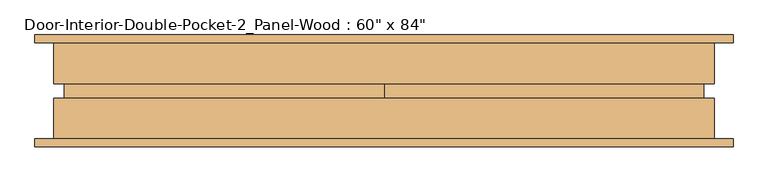
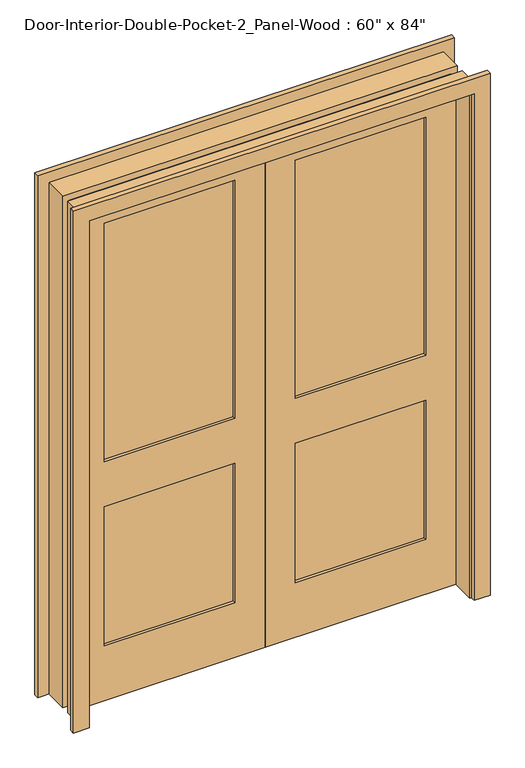
"""IFC4 building model written with IfcOpenShell, lengths in millimetres: door geometry."""

from ifc_helpers import new_model, si_unit, frame, origin, place, context, project, spatial, polyline, outline, extrude, source, transform, mapped, element, save


def door_53d589bd(model_context):
    return source(origin(), model_context, "Body", "SweptSolid", [
        extrude(outline(polyline([(0.0, 768.35), (0.0, 831.85), (2203.45, 831.85), (2203.45, -831.85), (0.0, -831.85), (0.0, -768.35), (2139.95, -768.35), (2139.95, 768.35), (0.0, 768.35)])), frame((0.0, -133.35, 0.0), z_axis=(0.0, 1.0, 0.0), x_axis=(0.0, 0.0, 1.0)), (0.0, 0.0, 1.0), 19.05),
        extrude(outline(polyline([(0.0, 768.35), (0.0, 831.85), (2203.45, 831.85), (2203.45, -831.85), (0.0, -831.85), (0.0, -768.35), (2139.95, -768.35), (2139.95, 768.35), (0.0, 768.35)])), frame((0.0, 114.3, 0.0), z_axis=(0.0, 1.0, 0.0), x_axis=(0.0, 0.0, 1.0)), (0.0, 0.0, 1.0), 19.05),
        extrude(outline(polyline([(-120.65, -5.8208333), (-641.35, -5.8208333), (-641.35, 5.8208333), (-120.65, 5.8208333), (-120.65, -5.8208333)])), frame((0.0, 0.0, 1009.65), z_axis=(0.0, 0.0, 1.0), x_axis=(1.0, 0.0, 0.0)), (0.0, 0.0, 1.0), 1004.8875),
        extrude(outline(polyline([(-120.65, -5.8208333), (-641.35, -5.8208333), (-641.35, 5.8208333), (-120.65, 5.8208333), (-120.65, -5.8208333)])), frame((0.0, 0.0, 231.775), z_axis=(0.0, 0.0, 1.0), x_axis=(1.0, 0.0, 0.0)), (0.0, 0.0, 1.0), 587.375),
        extrude(outline(polyline([(2133.6, -762.0), (0.0, -762.0), (0.0, 0.0), (2133.6, 0.0), (2133.6, -762.0)]), holes=[polyline([(2014.5375, -641.35), (2014.5375, -120.65), (1009.65, -120.65), (1009.65, -641.35), (2014.5375, -641.35)]), polyline([(819.15, -641.35), (819.15, -120.65), (231.775, -120.65), (231.775, -641.35), (819.15, -641.35)])]), frame((0.0, -17.4625, 0.0), z_axis=(0.0, 1.0, 0.0), x_axis=(0.0, 0.0, 1.0)), (0.0, 0.0, 1.0), 34.925),
        extrude(outline(polyline([(0.0, 787.4), (2159.0, 787.4), (2159.0, -787.4), (0.0, -787.4), (0.0, -762.0), (2133.6, -762.0), (2133.6, 762.0), (0.0, 762.0), (0.0, 787.4)])), frame((0.0, 17.4625, 0.0), z_axis=(0.0, 1.0, 0.0), x_axis=(0.0, 0.0, 1.0)), (0.0, 0.0, 1.0), 96.8375),
        extrude(outline(polyline([(0.0, 787.4), (2159.0, 787.4), (2159.0, -787.4), (0.0, -787.4), (0.0, -762.0), (2133.6, -762.0), (2133.6, 762.0), (0.0, 762.0), (0.0, 787.4)])), frame((0.0, -114.3, 0.0), z_axis=(0.0, 1.0, 0.0), x_axis=(0.0, 0.0, 1.0)), (0.0, 0.0, 1.0), 96.8375),
        extrude(outline(polyline([(641.35, -5.8208333), (120.65, -5.8208333), (120.65, 5.8208333), (641.35, 5.8208333), (641.35, -5.8208333)])), frame((0.0, 0.0, 1009.65), z_axis=(0.0, 0.0, 1.0), x_axis=(1.0, 0.0, 0.0)), (0.0, 0.0, 1.0), 1004.8875),
        extrude(outline(polyline([(641.35, -5.8208333), (120.65, -5.8208333), (120.65, 5.8208333), (641.35, 5.8208333), (641.35, -5.8208333)])), frame((0.0, 0.0, 231.775), z_axis=(0.0, 0.0, 1.0), x_axis=(1.0, 0.0, 0.0)), (0.0, 0.0, 1.0), 587.375),
        extrude(outline(polyline([(2133.6, 0.0), (0.0, 0.0), (0.0, 762.0), (2133.6, 762.0), (2133.6, 0.0)]), holes=[polyline([(2014.5375, 120.65), (2014.5375, 641.35), (1009.65, 641.35), (1009.65, 120.65), (2014.5375, 120.65)]), polyline([(819.15, 120.65), (819.15, 641.35), (231.775, 641.35), (231.775, 120.65), (819.15, 120.65)])]), frame((0.0, -17.4625, 0.0), z_axis=(0.0, 1.0, 0.0), x_axis=(0.0, 0.0, 1.0)), (0.0, 0.0, 1.0), 34.925),
    ])


if __name__ == "__main__":
    model = new_model("IFC4")
    model_context = context("Model", 3, world=origin())
    ifc_project = project(units=[si_unit("LENGTHUNIT", "METRE", prefix="MILLI")], contexts=[model_context])
    site = spatial("IfcSite", under=ifc_project)
    building = spatial("IfcBuilding", under=site)
    placement = place(None, origin())
    door_shape = door_53d589bd(model_context)
    element("IfcDoor", 1, ObjectType="Door-Interior-Double-Pocket-2_Panel-Wood : 60\" x 84\"", at=placement, inside=building, context=model_context, shape_type="MappedRepresentation", body=[
        mapped(door_shape, transform((0.0, 0.0, 0.0), x_axis=(1.0, 0.0, 0.0), y_axis=(0.0, 1.0, 0.0), z_axis=(0.0, 0.0, 1.0))),
    ])
    save(model, "model.ifc")

# Revit data of these elements
# Type "Door-Interior-Double-Pocket-2_Panel-Wood : 60\" x 84\""
#   Type Mark = "12"
#   Assembly Code = "C1020300"
#   Analytic Construction = "Wooden"
#   Top Rail = 0' - 4 11/16"
#   Thickness = 0' - 1 3/8"
#   Thermal Resistance (R) = 2.5876 (h·ft²·°F)/BTU
#   Stiles = 0' - 4 3/4"
#   Rough Width = 10' - 2"
#   Rough Height = 7' - 4 1/2"
#   Panel Width = 2' - 6"
#   Lock Rail = 0' - 7 1/2"
#   Location [instance default] = 2' - 7"
#   Height = 7' - 0"
#   Width = 5' - 0"
#   Heat Transfer Coefficient (U) = 0.3865 BTU/(h·ft²·°F)
#   Bottom Rail = 0' - 9 1/8"
#   Panel Open [instance default] = no
#   Trim Material = Cherry
#   Panel Material = Cherry
#   Frame Material = Cherry
#   Visual Light Transmittance = 0
#   Solar Heat Gain Coefficient = 0
#   Wall Closure = (empty or 0)
#   Function = (empty or 0)
# Element 1 (IfcDoor, "Door-Interior-Double-Pocket-2_Panel-Wood : 60\" x 84\"")
#   Materials on its faces: "Cherry"
# Materials
#   "Cherry": class "Wood", colour RGB 226 177 128, transparency 0, Description = "Prunus Serotina", Cost = 0
